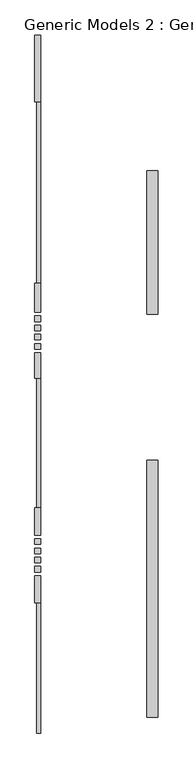
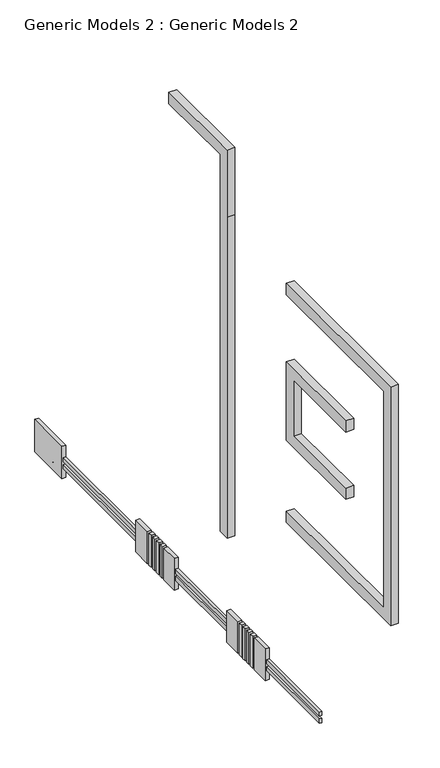
"""IFC4 building model written with IfcOpenShell, lengths in millimetres: proxy geometry, Generic Models 2 : Generic Models 2."""

from ifc_helpers import new_model, si_unit, frame, origin, place, context, project, spatial, polyline, circle_curve, outline, extrude, faceted_brep, source, transform, mapped, element, save
from ifc_brep_helpers import plane_surface, revolved_surface, advanced_brep


def generic_models_2_generic_models_2_d91b4525(model_context):
    return source(origin(), model_context, "Body", "SolidModel", [
        extrude(outline(polyline([(-10310.3415084, 5021.333346), (-10310.3415084, 9950.3230575), (-10208.7415084, 9950.3230575), (-10208.7415084, 5021.333346), (-10310.3415084, 5021.333346)])), frame((0.0, 0.0, 674.4572888), z_axis=(0.0, 0.0, 1.0), x_axis=(1.0, 0.0, 0.0)), (0.0, 0.0, 1.0), 163.7427112),
        extrude(outline(polyline([(-10310.3415084, 5021.333346), (-10310.3415084, 9950.3230575), (-10208.7415084, 9950.3230575), (-10208.7415084, 5021.333346), (-10310.3415084, 5021.333346)])), frame((0.0, 0.0, 378.5350621), z_axis=(0.0, 0.0, 1.0), x_axis=(1.0, 0.0, 0.0)), (0.0, 0.0, 1.0), 180.2649379),
        extrude(outline(polyline([(-1074.666654, 838.2), (2445.1720575, 838.2), (2445.1720575, 674.4572888), (-1074.117654, 674.4572888), (-1074.117654, 558.8), (2445.1720575, 558.8), (2445.1720575, 378.5350621), (-1074.666654, 378.5350621), (-1074.666654, 838.2)])), frame((-10310.3415084, 0.0, 0.0), z_axis=(1.0, 0.0, 0.0), x_axis=(0.0, 1.0, 0.0)), (0.0, 0.0, 1.0), 101.6),
        extrude(outline(polyline([(-10310.3415084, -7182.817654), (-10310.3415084, -3650.8279425), (-10208.7415084, -3650.8279425), (-10208.7415084, -7182.817654), (-10310.3415084, -7182.817654)])), frame((0.0, 0.0, 674.4572888), z_axis=(0.0, 0.0, 1.0), x_axis=(1.0, 0.0, 0.0)), (0.0, 0.0, 1.0), 163.7427112),
        extrude(outline(polyline([(-10310.3415084, -7182.817654), (-10310.3415084, -3650.8279425), (-10208.7415084, -3650.8279425), (-10208.7415084, -7182.817654), (-10310.3415084, -7182.817654)])), frame((0.0, 0.0, 378.5350621), z_axis=(0.0, 0.0, 1.0), x_axis=(1.0, 0.0, 0.0)), (0.0, 0.0, 1.0), 180.2649379),
        advanced_brep(
        [(-10361.1415084, 9950.3230575, 1320.8), (-10361.1415084, 11758.4890135, 1320.8), (-10361.1415084, 11758.4890135, 0.0), (-10361.1415084, 9950.3230575, 0.0), (-10208.7415084, 9950.3230575, 0.0), (-10208.7415084, 11758.4890135, 0.0), (-10208.7415084, 11758.4890135, 1320.8), (-10208.7415084, 9950.3230575, 1320.8), (-10208.7415084, 9950.3230575, 674.4572888), (-10208.7415084, 9950.3230575, 558.8), (-10208.7415084, 11346.9481892, 623.6572888), (-10208.7415084, 10432.5481892, 623.6572888), (-10310.3415084, 10432.5481892, 623.6572888), (-10310.3415084, 11346.9481892, 623.6572888)],
        [
            (0, 1),
            (1, 2),
            (2, 3),
            (3, 0),
            (4, 5),
            (5, 6),
            (6, 7),
            (7, 8),
            (8, 9),
            (9, 4),
            (10, 11, circle_curve(frame((-10208.7415084, 10889.7481892, 623.6572888), z_axis=(-1.0, 0.0, 0.0), x_axis=(0.0, 1.0, 0.0)), 457.2)),
            (11, 10, circle_curve(frame((-10208.7415084, 10889.7481892, 623.6572888), z_axis=(-1.0, 0.0, 0.0), x_axis=(0.0, 1.0, 0.0)), 457.2)),
            (0, 7),
            (6, 1),
            (5, 2),
            (4, 3),
            (12, 13, circle_curve(frame((-10310.3415084, 10889.7481892, 623.6572888), z_axis=(1.0, 0.0, 0.0), x_axis=(0.0, 1.0, 0.0)), 457.2)),
            (13, 12, circle_curve(frame((-10310.3415084, 10889.7481892, 623.6572888), z_axis=(1.0, 0.0, 0.0), x_axis=(0.0, 1.0, 0.0)), 457.2)),
            (13, 10),
            (11, 12),
        ],
        [
            plane_surface(frame((-10361.1415084, 11758.4890135, 1320.8), z_axis=(-1.0, 0.0, 0.0), x_axis=(0.0, 1.0, 0.0))),
            plane_surface(frame((-10208.7415084, 11758.4890135, 1320.8), z_axis=(1.0, 0.0, 0.0), x_axis=(0.0, -1.0, 0.0))),
            plane_surface(frame((-10361.1415084, 9950.3230575, 1320.8), z_axis=(0.0, 0.0, 1.0), x_axis=(1.0, 0.0, 0.0))),
            plane_surface(frame((-10361.1415084, 11758.4890135, 1320.8), z_axis=(0.0, 1.0, 0.0), x_axis=(1.0, 0.0, 0.0))),
            plane_surface(frame((-10361.1415084, 11758.4890135, 0.0), z_axis=(0.0, 0.0, -1.0), x_axis=(1.0, 0.0, 0.0))),
            plane_surface(frame((-10361.1415084, 9950.3230575, 0.0), z_axis=(0.0, -1.0, 0.0), x_axis=(1.0, 0.0, 0.0))),
            plane_surface(frame((-10310.3415084, 9950.3230575, 558.8), z_axis=(1.0, 0.0, 0.0), x_axis=(0.0, -1.0, 0.0))),
            revolved_surface(polyline([(-10208.7415084, 11346.9481892, 623.6572888), (-10310.3415084, 11346.9481892, 623.6572888)]), (-10310.3415084, 10889.7481892, 623.6572888), (1.0, 0.0, 0.0)),
        ],
        [
            (0, [[1, 2, 3, 4]]),
            (1, [[5, 6, 7, 8, 9, 10], [11, 12]]),
            (2, [[-1, 13, -7, 14]]),
            (3, [[-2, -14, -6, 15]]),
            (4, [[-3, -15, -5, 16]]),
            (5, [[-4, -16, -10, -9, -8, -13]]),
            (6, [[17, 18]]),
            (7, [[-18, 19, -12, 20]]),
            (7, [[-17, -20, -11, -19]]),
        ],
    ),
        faceted_brep([(-10361.1415084, 5021.333346, 1298.1145776), (-10361.1415084, 5021.333346, 0.0), (-10361.1415084, 4232.5534, 0.0), (-10361.1415084, 4232.5534, 1298.1145776), (-10208.7415084, 4232.5534, 0.0), (-10208.7415084, 5021.333346, 0.0), (-10208.7415084, 5021.333346, 558.8), (-10208.7415084, 5021.333346, 674.4572888), (-10208.7415084, 5021.333346, 1298.1145776), (-10208.7415084, 4232.5534, 1298.1145776)], [[[0, 1, 2, 3]], [[4, 5, 6, 7, 8, 9]], [[8, 0, 3, 9]], [[1, 0, 8, 7, 6, 5]], [[1, 5, 4, 2]], [[3, 2, 4, 9]]]),
        faceted_brep([(-10361.1415084, 2445.1720575, 0.0), (-10361.1415084, 2445.1720575, 1298.1145776), (-10361.1415084, 3136.7016544, 1298.1145776), (-10361.1415084, 3136.7016544, 0.0), (-10208.7415084, 2445.1720575, 0.0), (-10208.7415084, 3136.7016544, 0.0), (-10208.7415084, 3136.7016544, 1298.1145776), (-10208.7415084, 2445.1720575, 1298.1145776), (-10208.7415084, 2445.1720575, 674.4572888), (-10208.7415084, 2445.1720575, 558.8)], [[[0, 1, 2, 3]], [[4, 5, 6, 7, 8, 9]], [[1, 7, 6, 2]], [[4, 0, 3, 5]], [[1, 0, 4, 9, 8, 7]], [[3, 2, 6, 5]]]),
        faceted_brep([(-10361.1415084, -1074.666654, 1298.1145776), (-10361.1415084, -1074.666654, 0.0), (-10361.1415084, -1814.8214255, 0.0), (-10361.1415084, -1814.8214255, 1298.1145776), (-10208.7415084, -1074.666654, 0.0), (-10208.7415084, -1074.666654, 1298.1145776), (-10208.7415084, -1814.8214255, 1298.1145776), (-10208.7415084, -1814.8214255, 0.0)], [[[0, 1, 2, 3]], [[4, 5, 6, 7]], [[5, 0, 3, 6]], [[1, 0, 5, 4]], [[1, 4, 7, 2]], [[3, 2, 7, 6]]]),
        faceted_brep([(-10361.1415084, -3650.8279425, 0.0), (-10361.1415084, -3650.8279425, 1298.1145776), (-10361.1415084, -2910.673171, 1298.1145776), (-10361.1415084, -2910.673171, 0.0), (-10208.7415084, -3650.8279425, 0.0), (-10208.7415084, -2910.673171, 0.0), (-10208.7415084, -2910.673171, 1298.1145776), (-10208.7415084, -3650.8279425, 1298.1145776), (-10208.7415084, -3650.8279425, 674.4572888), (-10208.7415084, -3650.8279425, 558.8)], [[[0, 1, 2, 3]], [[4, 5, 6, 7, 8, 9]], [[1, 7, 6, 2]], [[4, 0, 3, 5]], [[1, 0, 4, 9, 8, 7]], [[3, 2, 6, 5]]]),
        faceted_brep([(-10361.1415084, 3483.6023526, 1298.1145776), (-10361.1415084, 3636.0023526, 1298.1145776), (-10361.1415084, 3636.0023526, 0.0), (-10361.1415084, 3483.6023526, 0.0), (-10208.7415084, 3483.6023526, 0.0), (-10208.7415084, 3636.0023526, 0.0), (-10208.7415084, 3636.0023526, 1298.1145776), (-10208.7415084, 3483.6023526, 1298.1145776)], [[[0, 1, 2, 3]], [[4, 5, 6, 7]], [[1, 0, 7, 6]], [[3, 2, 5, 4]], [[2, 1, 6, 5]], [[0, 3, 4, 7]]]),
        faceted_brep([(-10361.1415084, 3733.2527017, 1298.1145776), (-10361.1415084, 3885.6527017, 1298.1145776), (-10361.1415084, 3885.6527017, 0.0), (-10361.1415084, 3733.2527017, 0.0), (-10208.7415084, 3733.2527017, 0.0), (-10208.7415084, 3885.6527017, 0.0), (-10208.7415084, 3885.6527017, 1298.1145776), (-10208.7415084, 3733.2527017, 1298.1145776)], [[[0, 1, 2, 3]], [[4, 5, 6, 7]], [[1, 0, 7, 6]], [[3, 2, 5, 4]], [[0, 3, 4, 7]], [[2, 1, 6, 5]]]),
        faceted_brep([(-10361.1415084, 3233.9520035, 1298.1145776), (-10361.1415084, 3386.3520035, 1298.1145776), (-10361.1415084, 3386.3520035, 0.0), (-10361.1415084, 3233.9520035, 0.0), (-10208.7415084, 3233.9520035, 0.0), (-10208.7415084, 3386.3520035, 0.0), (-10208.7415084, 3386.3520035, 1298.1145776), (-10208.7415084, 3233.9520035, 1298.1145776)], [[[0, 1, 2, 3]], [[4, 5, 6, 7]], [[1, 0, 7, 6]], [[3, 2, 5, 4]], [[2, 1, 6, 5]], [[0, 3, 4, 7]]]),
        faceted_brep([(-10361.1415084, 3982.9030509, 1298.1145776), (-10361.1415084, 4135.3030509, 1298.1145776), (-10361.1415084, 4135.3030509, 0.0), (-10361.1415084, 3982.9030509, 0.0), (-10208.7415084, 3982.9030509, 0.0), (-10208.7415084, 4135.3030509, 0.0), (-10208.7415084, 4135.3030509, 1298.1145776), (-10208.7415084, 3982.9030509, 1298.1145776)], [[[0, 1, 2, 3]], [[4, 5, 6, 7]], [[1, 0, 7, 6]], [[3, 2, 5, 4]], [[0, 3, 4, 7]], [[2, 1, 6, 5]]]),
        faceted_brep([(-10361.1415084, -2563.7724728, 1298.1145776), (-10361.1415084, -2411.3724728, 1298.1145776), (-10361.1415084, -2411.3724728, 0.0), (-10361.1415084, -2563.7724728, 0.0), (-10208.7415084, -2563.7724728, 0.0), (-10208.7415084, -2411.3724728, 0.0), (-10208.7415084, -2411.3724728, 1298.1145776), (-10208.7415084, -2563.7724728, 1298.1145776)], [[[0, 1, 2, 3]], [[4, 5, 6, 7]], [[1, 0, 7, 6]], [[3, 2, 5, 4]], [[2, 1, 6, 5]], [[0, 3, 4, 7]]]),
        faceted_brep([(-10361.1415084, -2314.1221237, 1298.1145776), (-10361.1415084, -2161.7221237, 1298.1145776), (-10361.1415084, -2161.7221237, 0.0), (-10361.1415084, -2314.1221237, 0.0), (-10208.7415084, -2314.1221237, 0.0), (-10208.7415084, -2161.7221237, 0.0), (-10208.7415084, -2161.7221237, 1298.1145776), (-10208.7415084, -2314.1221237, 1298.1145776)], [[[0, 1, 2, 3]], [[4, 5, 6, 7]], [[1, 0, 7, 6]], [[3, 2, 5, 4]], [[0, 3, 4, 7]], [[2, 1, 6, 5]]]),
        faceted_brep([(-10361.1415084, -2813.4228219, 1298.1145776), (-10361.1415084, -2661.0228219, 1298.1145776), (-10361.1415084, -2661.0228219, 0.0), (-10361.1415084, -2813.4228219, 0.0), (-10208.7415084, -2813.4228219, 0.0), (-10208.7415084, -2661.0228219, 0.0), (-10208.7415084, -2661.0228219, 1298.1145776), (-10208.7415084, -2813.4228219, 1298.1145776)], [[[0, 1, 2, 3]], [[4, 5, 6, 7]], [[1, 0, 7, 6]], [[3, 2, 5, 4]], [[2, 1, 6, 5]], [[0, 3, 4, 7]]]),
        faceted_brep([(-10361.1415084, -2064.4717746, 1298.1145776), (-10361.1415084, -1912.0717746, 1298.1145776), (-10361.1415084, -1912.0717746, 0.0), (-10361.1415084, -2064.4717746, 0.0), (-10208.7415084, -2064.4717746, 0.0), (-10208.7415084, -1912.0717746, 0.0), (-10208.7415084, -1912.0717746, 1298.1145776), (-10208.7415084, -2064.4717746, 1298.1145776)], [[[0, 1, 2, 3]], [[4, 5, 6, 7]], [[1, 0, 7, 6]], [[3, 2, 5, 4]], [[0, 3, 4, 7]], [[2, 1, 6, 5]]]),
        extrude(outline(polyline([(4183.133346, 15849.6), (8069.333346, 15849.6), (8069.333346, 15392.4), (4640.333346, 15392.4), (4640.333346, 0.0), (4183.133346, 0.0), (4183.133346, 13106.4), (4183.133346, 15849.6)])), frame((-7313.1415084, 0.0, 0.0), z_axis=(1.0, 0.0, 0.0), x_axis=(0.0, 1.0, 0.0)), (0.0, 0.0, 1.0), 304.8),
        extrude(outline(polyline([(-6751.566654, 12801.6), (223.273346, 12801.6), (223.273346, 12344.4), (-6294.366654, 12344.4), (-6294.366654, 3505.2), (220.733346, 3505.2), (220.733346, 3048.0), (-6751.566654, 3048.0), (-6751.566654, 12801.6)])), frame((-7313.1415084, 0.0, 0.0), z_axis=(1.0, 0.0, 0.0), x_axis=(0.0, 1.0, 0.0)), (0.0, 0.0, 1.0), 304.8),
        extrude(outline(polyline([(220.733346, 9601.2), (220.733346, 6400.8), (-3751.826654, 6400.8), (-3751.826654, 6858.0), (-261.866654, 6858.0), (-261.866654, 9144.0), (-2636.766654, 9144.0), (-3751.826654, 9144.0), (-3751.826654, 9601.2), (220.733346, 9601.2)])), frame((-7313.1415084, 0.0, 0.0), z_axis=(1.0, 0.0, 0.0), x_axis=(0.0, 1.0, 0.0)), (0.0, 0.0, 1.0), 304.8),
    ])


if __name__ == "__main__":
    model = new_model("IFC4")
    model_context = context("Model", 3, world=origin())
    ifc_project = project(units=[si_unit("LENGTHUNIT", "METRE", prefix="MILLI")], contexts=[model_context])
    site = spatial("IfcSite", under=ifc_project)
    building = spatial("IfcBuilding", under=site)
    placement = place(None, origin())
    generic_models_2_generic_models_2_shape = generic_models_2_generic_models_2_d91b4525(model_context)
    element("IfcBuildingElementProxy", 1, Name="Generic Models 2 : Generic Models 2", ObjectType="Generic Models 2 : Generic Models 2", at=placement, inside=building, context=model_context, shape_type="MappedRepresentation", body=[
        mapped(generic_models_2_generic_models_2_shape, transform((0.0, 0.0, 0.0), x_axis=(1.0, 0.0, 0.0), y_axis=(0.0, 1.0, 0.0), z_axis=(0.0, 0.0, 1.0))),
    ])
    save(model, "model.ifc")

# Revit data of these elements
# Element 1 (IfcBuildingElementProxy, "Generic Models 2 : Generic Models 2")
#   Materials on its faces: "Wood Planks", "GATE"
# Materials
#   "Wood Planks": class "Wood", colour RGB 193 160 115, transparency 0, Description = "Physical material.", Cost = 0
#   "GATE": class "Generic", colour RGB 120 120 120, transparency 0, Cost = 0
